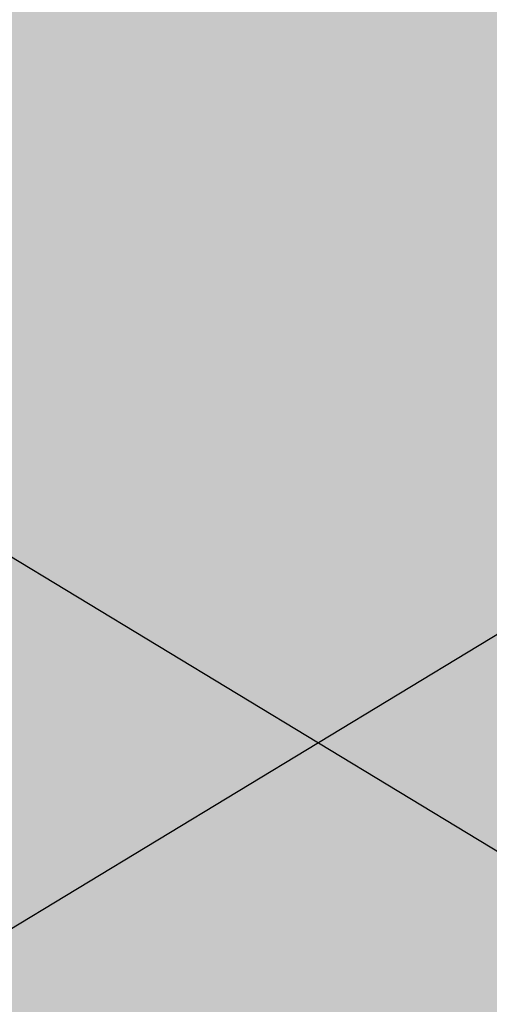
# Model space of a CAD drawing. Units: millimetres. Extents: x -22994 to 29398, y -19990 to 20176.
# Tile 59 of 135: x 215.97 to 223.11, y 79.59 to 94.56. Entities that reach past the tile are written whole.
import ezdxf
from ezdxf import colors
from ezdxf.entities.mleader import LeaderData, LeaderLine
from ezdxf.math import Vec2, Vec3

# ---------------------------------------------------------------- set-up
doc = ezdxf.new("R2010")
doc.units = ezdxf.units.MM
doc.header["$MEASUREMENT"] = 0
for name, color, linetype, lineweight in [('M-ANNO-TEXT', 7, 'Continuous', 25), ('M-DIMS', 2, 'Continuous', 18), ('M-EQPM', 7, 'Continuous', 25), ('M-EQPM-PATT', 7, 'Continuous', 18)]:
    doc.layers.add(name, color=color, linetype=linetype, lineweight=lineweight)
doc.styles.get("Standard").update_dxf_attribs({"font": 'arial.ttf'})
doc.dimstyles.get("Standard").update_dxf_attribs({"dimtxt": 0.18, "dimasz": 10000, "dimexe": 0.18, "dimexo": 0.0625, "dimgap": 0.09, "dimtad": 0, "dimtih": 1, "dimtoh": 1, "dimdec": 0, "dimzin": 0, "dimdsep": 46, "dimtxsty": 'Standard', "dimcen": 0.09, "dimadec": 0, "dimazin": 0, "dimtfac": 1, "dimtdec": 0, "dimtofl": 0, "dimtmove": 0, "dimatfit": 3, "dimfxl": 1, "dimtolj": 1, "dimtzin": 0, "dimlwd": 30, "dimarcsym": 0})

# ---------------------------------------------------------------- blocks, each defined once
blk = doc.blocks.new('*D2')
at = {"layer": 'Defpoints', "color": 0, "transparency": 16777216}
for p in [(6.677, 10.271), (290.852, 10.271), (290.852, -5.079)]:
    blk.add_point(p, dxfattribs=at)
at = {"layer": 'M-DIMS', "color": 0, "lineweight": -2, "transparency": 16777216}
for p, q in [((6.677, 10.209), (6.677, -5.259)), ((290.852, 10.209), (290.852, -5.259))]:
    blk.add_line(p, q, dxfattribs=at)
at = {"layer": 'M-DIMS', "color": 0, "lineweight": 30, "transparency": 16777216}
for p, q in [((-9993.323, -5.079), (-19993.323, -5.079)), ((10290.852, -5.079), (20290.852, -5.079))]:
    blk.add_line(p, q, dxfattribs=at)
at = {"layer": 'M-DIMS', "color": 0, "transparency": 16777216}
for points in [[(-9993.323, 1661.588), (-9993.323, -1671.745), (6.677, -5.079)], [(10290.852, 1661.588), (10290.852, -1671.745), (290.852, -5.079)]]:
    blk.add_solid(points, dxfattribs=at)
at = {"layer": 'M-DIMS', "color": 0, "transparency": 16777216, "insert": (148.765, -5.079), "char_height": 0.18, "attachment_point": 5}
blk.add_mtext('\\A1;284.2', dxfattribs=at)
blk = doc.blocks.new('*D3')
at = {"layer": 'Defpoints', "color": 0, "transparency": 16777216}
for p in [(110.265, 204.165), (110.265, 176.366), (95.833, 127.967)]:
    blk.add_point(p, dxfattribs=at)
at = {"layer": 'M-DIMS', "color": 0, "lineweight": -2, "transparency": 16777216}
for p, q in [((95.833, 128.03), (95.833, 204.345)), ((110.265, 176.429), (110.265, 204.345))]:
    blk.add_line(p, q, dxfattribs=at)
at = {"layer": 'M-DIMS', "color": 0, "lineweight": 30, "transparency": 16777216}
for p, q in [((-9904.167, 204.165), (-19904.167, 204.165)), ((10110.265, 204.165), (20110.265, 204.165))]:
    blk.add_line(p, q, dxfattribs=at)
at = {"layer": 'M-DIMS', "color": 0, "transparency": 16777216}
for points in [[(-9904.167, 1870.832), (-9904.167, -1462.501), (95.833, 204.165)], [(10110.265, 1870.832), (10110.265, -1462.501), (110.265, 204.165)]]:
    blk.add_solid(points, dxfattribs=at)
at = {"layer": 'M-DIMS', "color": 0, "transparency": 16777216, "insert": (103.049, 204.165), "char_height": 0.18, "attachment_point": 5}
blk.add_mtext('\\A1;14.432', dxfattribs=at)
blk = doc.blocks.new('*D4')
at = {"layer": 'Defpoints', "color": 0, "transparency": 16777216}
for p in [(116.265, 204.165), (110.265, 176.366), (116.265, 176.366)]:
    blk.add_point(p, dxfattribs=at)
at = {"layer": 'M-DIMS', "color": 0, "lineweight": -2, "transparency": 16777216}
for p, q in [((110.265, 176.429), (110.265, 204.345)), ((116.265, 176.429), (116.265, 204.345))]:
    blk.add_line(p, q, dxfattribs=at)
at = {"layer": 'M-DIMS', "color": 0, "lineweight": 30, "transparency": 16777216}
for p, q in [((-9889.735, 204.165), (-19889.735, 204.165)), ((10116.265, 204.165), (20116.265, 204.165))]:
    blk.add_line(p, q, dxfattribs=at)
at = {"layer": 'M-DIMS', "color": 0, "transparency": 16777216}
for points in [[(-9889.735, 1870.832), (-9889.735, -1462.501), (110.265, 204.165)], [(10116.265, 1870.832), (10116.265, -1462.501), (116.265, 204.165)]]:
    blk.add_solid(points, dxfattribs=at)
at = {"layer": 'M-DIMS', "color": 0, "transparency": 16777216, "insert": (113.265, 204.165), "char_height": 0.18, "attachment_point": 5}
blk.add_mtext('\\A1;6', dxfattribs=at)
blk = doc.blocks.new('*D5')
at = {"layer": 'Defpoints', "color": 0, "transparency": 16777216}
for p in [(181.265, 204.165), (116.265, 176.366), (181.265, 176.366)]:
    blk.add_point(p, dxfattribs=at)
at = {"layer": 'M-DIMS', "color": 0, "lineweight": -2, "transparency": 16777216}
for p, q in [((116.265, 176.429), (116.265, 204.345)), ((181.265, 176.429), (181.265, 204.345))]:
    blk.add_line(p, q, dxfattribs=at)
at = {"layer": 'M-DIMS', "color": 0, "lineweight": 30, "transparency": 16777216}
for p, q in [((-9883.735, 204.165), (-19883.735, 204.165)), ((10181.265, 204.165), (20181.265, 204.165))]:
    blk.add_line(p, q, dxfattribs=at)
at = {"layer": 'M-DIMS', "color": 0, "transparency": 16777216}
for points in [[(-9883.735, 1870.832), (-9883.735, -1462.501), (116.265, 204.165)], [(10181.265, 1870.832), (10181.265, -1462.501), (181.265, 204.165)]]:
    blk.add_solid(points, dxfattribs=at)
at = {"layer": 'M-DIMS', "color": 0, "transparency": 16777216, "insert": (148.765, 204.165), "char_height": 0.18, "attachment_point": 5}
blk.add_mtext('\\A1;65', dxfattribs=at)
blk = doc.blocks.new('*D6')
at = {"layer": 'Defpoints', "color": 0, "transparency": 16777216}
for p in [(187.265, 204.165), (181.265, 176.366), (187.265, 176.366)]:
    blk.add_point(p, dxfattribs=at)
at = {"layer": 'M-DIMS', "color": 0, "lineweight": -2, "transparency": 16777216}
for p, q in [((181.265, 176.429), (181.265, 204.345)), ((187.265, 176.429), (187.265, 204.345))]:
    blk.add_line(p, q, dxfattribs=at)
at = {"layer": 'M-DIMS', "color": 0, "lineweight": 30, "transparency": 16777216}
for p, q in [((-9818.735, 204.165), (-19818.735, 204.165)), ((10187.265, 204.165), (20187.265, 204.165))]:
    blk.add_line(p, q, dxfattribs=at)
at = {"layer": 'M-DIMS', "color": 0, "transparency": 16777216}
for points in [[(-9818.735, 1870.832), (-9818.735, -1462.501), (181.265, 204.165)], [(10187.265, 1870.832), (10187.265, -1462.501), (187.265, 204.165)]]:
    blk.add_solid(points, dxfattribs=at)
at = {"layer": 'M-DIMS', "color": 0, "transparency": 16777216, "insert": (184.265, 204.165), "char_height": 0.18, "attachment_point": 5}
blk.add_mtext('\\A1;6', dxfattribs=at)
blk = doc.blocks.new('*D7')
at = {"layer": 'Defpoints', "color": 0, "transparency": 16777216}
for p in [(201.697, 204.165), (187.265, 176.366), (201.697, 127.967)]:
    blk.add_point(p, dxfattribs=at)
at = {"layer": 'M-DIMS', "color": 0, "lineweight": -2, "transparency": 16777216}
for p, q in [((187.265, 176.429), (187.265, 204.345)), ((201.697, 128.03), (201.697, 204.345))]:
    blk.add_line(p, q, dxfattribs=at)
at = {"layer": 'M-DIMS', "color": 0, "lineweight": 30, "transparency": 16777216}
for p, q in [((-9812.735, 204.165), (-19812.735, 204.165)), ((10201.697, 204.165), (20201.697, 204.165))]:
    blk.add_line(p, q, dxfattribs=at)
at = {"layer": 'M-DIMS', "color": 0, "transparency": 16777216}
for points in [[(-9812.735, 1870.832), (-9812.735, -1462.501), (187.265, 204.165)], [(10201.697, 1870.832), (10201.697, -1462.501), (201.697, 204.165)]]:
    blk.add_solid(points, dxfattribs=at)
at = {"layer": 'M-DIMS', "color": 0, "transparency": 16777216, "insert": (194.481, 204.165), "char_height": 0.18, "attachment_point": 5}
blk.add_mtext('\\A1;14.432', dxfattribs=at)
blk = doc.blocks.new('*D8')
at = {"layer": 'Defpoints', "color": 0, "transparency": 16777216}
for p in [(227.648, 204.165), (227.648, 146.73), (201.697, 127.967)]:
    blk.add_point(p, dxfattribs=at)
at = {"layer": 'M-DIMS', "color": 0, "lineweight": -2, "transparency": 16777216}
for p, q in [((201.697, 128.03), (201.697, 204.345)), ((227.648, 146.792), (227.648, 204.345))]:
    blk.add_line(p, q, dxfattribs=at)
at = {"layer": 'M-DIMS', "color": 0, "lineweight": 30, "transparency": 16777216}
for p, q in [((-9798.303, 204.165), (-19798.303, 204.165)), ((10227.648, 204.165), (20227.648, 204.165))]:
    blk.add_line(p, q, dxfattribs=at)
at = {"layer": 'M-DIMS', "color": 0, "transparency": 16777216}
for points in [[(-9798.303, 1870.832), (-9798.303, -1462.501), (201.697, 204.165)], [(10227.648, 1870.832), (10227.648, -1462.501), (227.648, 204.165)]]:
    blk.add_solid(points, dxfattribs=at)
at = {"layer": 'M-DIMS', "color": 0, "transparency": 16777216, "insert": (214.673, 204.165), "char_height": 0.18, "attachment_point": 5}
blk.add_mtext('\\A1;25.95', dxfattribs=at)
blk = doc.blocks.new('*D9')
at = {"layer": 'Defpoints', "color": 0, "transparency": 16777216}
for p in [(187.265, 176.366), (306.202, 176.366), (290.852, 10.271)]:
    blk.add_point(p, dxfattribs=at)
at = {"layer": 'M-DIMS', "color": 0, "lineweight": 30, "transparency": 16777216}
for p, q in [((306.202, 10176.366), (306.202, 20176.366)), ((306.202, -9989.729), (306.202, -19989.729))]:
    blk.add_line(p, q, dxfattribs=at)
at = {"layer": 'M-DIMS', "color": 0, "lineweight": -2, "transparency": 16777216}
for p, q in [((187.327, 176.366), (306.382, 176.366)), ((290.915, 10.271), (306.382, 10.271))]:
    blk.add_line(p, q, dxfattribs=at)
at = {"layer": 'M-DIMS', "color": 0, "transparency": 16777216}
for points in [[(-1360.465, 10176.366), (1972.869, 10176.366), (306.202, 176.366)], [(-1360.465, -9989.729), (1972.869, -9989.729), (306.202, 10.271)]]:
    blk.add_solid(points, dxfattribs=at)
at = {"layer": 'M-DIMS', "color": 0, "transparency": 16777216, "insert": (306.202, 93.319), "char_height": 0.18, "attachment_point": 5}
blk.add_mtext('\\A1;166.1', dxfattribs=at)
blk = doc.blocks.new('*D10')
at = {"layer": 'Defpoints', "color": 0, "transparency": 16777216}
for p in [(125.65, 136.071), (133.346, 136.071), (133.346, -5.079)]:
    blk.add_point(p, dxfattribs=at)
at = {"layer": 'M-DIMS', "color": 0, "lineweight": -2, "transparency": 16777216}
for p, q in [((125.65, 136.009), (125.65, -5.259)), ((133.346, 136.009), (133.346, -5.259))]:
    blk.add_line(p, q, dxfattribs=at)
at = {"layer": 'M-DIMS', "color": 0, "lineweight": 30, "transparency": 16777216}
for p, q in [((-9874.35, -5.079), (-19874.35, -5.079)), ((10133.346, -5.079), (20133.346, -5.079))]:
    blk.add_line(p, q, dxfattribs=at)
at = {"layer": 'M-DIMS', "color": 0, "transparency": 16777216}
for points in [[(-9874.35, 1661.588), (-9874.35, -1671.745), (125.65, -5.079)], [(10133.346, 1661.588), (10133.346, -1671.745), (133.346, -5.079)]]:
    blk.add_solid(points, dxfattribs=at)
at = {"layer": 'M-DIMS', "color": 0, "transparency": 16777216, "insert": (129.498, -5.079), "char_height": 0.18, "attachment_point": 5}
blk.add_mtext('\\A1;7.696', dxfattribs=at)
blk = doc.blocks.new('*D11')
at = {"layer": 'Defpoints', "color": 0, "transparency": 16777216}
for p in [(133.346, 136.071), (135.65, 136.071), (135.65, -5.079)]:
    blk.add_point(p, dxfattribs=at)
at = {"layer": 'M-DIMS', "color": 0, "lineweight": -2, "transparency": 16777216}
for p, q in [((133.346, 136.009), (133.346, -5.259)), ((135.65, 136.009), (135.65, -5.259))]:
    blk.add_line(p, q, dxfattribs=at)
at = {"layer": 'M-DIMS', "color": 0, "lineweight": 30, "transparency": 16777216}
for p, q in [((-9866.654, -5.079), (-19866.654, -5.079)), ((10135.65, -5.079), (20135.65, -5.079))]:
    blk.add_line(p, q, dxfattribs=at)
at = {"layer": 'M-DIMS', "color": 0, "transparency": 16777216}
for points in [[(-9866.654, 1661.588), (-9866.654, -1671.745), (133.346, -5.079)], [(10135.65, 1661.588), (10135.65, -1671.745), (135.65, -5.079)]]:
    blk.add_solid(points, dxfattribs=at)
at = {"layer": 'M-DIMS', "color": 0, "transparency": 16777216, "insert": (134.498, -5.079), "char_height": 0.18, "attachment_point": 5}
blk.add_mtext('\\A1;2.304', dxfattribs=at)
blk = doc.blocks.new('*D12')
at = {"layer": 'Defpoints', "color": 0, "transparency": 16777216}
for p in [(135.65, 136.071), (145.65, 136.071), (145.65, -5.079)]:
    blk.add_point(p, dxfattribs=at)
at = {"layer": 'M-DIMS', "color": 0, "lineweight": -2, "transparency": 16777216}
for p, q in [((135.65, 136.009), (135.65, -5.259)), ((145.65, 136.009), (145.65, -5.259))]:
    blk.add_line(p, q, dxfattribs=at)
at = {"layer": 'M-DIMS', "color": 0, "lineweight": 30, "transparency": 16777216}
for p, q in [((-9864.35, -5.079), (-19864.35, -5.079)), ((10145.65, -5.079), (20145.65, -5.079))]:
    blk.add_line(p, q, dxfattribs=at)
at = {"layer": 'M-DIMS', "color": 0, "transparency": 16777216}
for points in [[(-9864.35, 1661.588), (-9864.35, -1671.745), (135.65, -5.079)], [(10145.65, 1661.588), (10145.65, -1671.745), (145.65, -5.079)]]:
    blk.add_solid(points, dxfattribs=at)
at = {"layer": 'M-DIMS', "color": 0, "transparency": 16777216, "insert": (140.65, -5.079), "char_height": 0.18, "attachment_point": 5}
blk.add_mtext('\\A1;10', dxfattribs=at)
blk = doc.blocks.new('*D13')
at = {"layer": 'Defpoints', "color": 0, "transparency": 16777216}
for p in [(145.65, 136.071), (155.65, 136.071), (155.65, -5.079)]:
    blk.add_point(p, dxfattribs=at)
at = {"layer": 'M-DIMS', "color": 0, "lineweight": -2, "transparency": 16777216}
for p, q in [((145.65, 136.009), (145.65, -5.259)), ((155.65, 136.009), (155.65, -5.259))]:
    blk.add_line(p, q, dxfattribs=at)
at = {"layer": 'M-DIMS', "color": 0, "lineweight": 30, "transparency": 16777216}
for p, q in [((-9854.35, -5.079), (-19854.35, -5.079)), ((10155.65, -5.079), (20155.65, -5.079))]:
    blk.add_line(p, q, dxfattribs=at)
at = {"layer": 'M-DIMS', "color": 0, "transparency": 16777216}
for points in [[(-9854.35, 1661.588), (-9854.35, -1671.745), (145.65, -5.079)], [(10155.65, 1661.588), (10155.65, -1671.745), (155.65, -5.079)]]:
    blk.add_solid(points, dxfattribs=at)
at = {"layer": 'M-DIMS', "color": 0, "transparency": 16777216, "insert": (150.65, -5.079), "char_height": 0.18, "attachment_point": 5}
blk.add_mtext('\\A1;10', dxfattribs=at)
blk = doc.blocks.new('*D14')
at = {"layer": 'Defpoints', "color": 0, "transparency": 16777216}
for p in [(155.65, 136.071), (165.65, 136.071), (165.65, -5.079)]:
    blk.add_point(p, dxfattribs=at)
at = {"layer": 'M-DIMS', "color": 0, "lineweight": -2, "transparency": 16777216}
for p, q in [((155.65, 136.009), (155.65, -5.259)), ((165.65, 136.009), (165.65, -5.259))]:
    blk.add_line(p, q, dxfattribs=at)
at = {"layer": 'M-DIMS', "color": 0, "lineweight": 30, "transparency": 16777216}
for p, q in [((-9844.35, -5.079), (-19844.35, -5.079)), ((10165.65, -5.079), (20165.65, -5.079))]:
    blk.add_line(p, q, dxfattribs=at)
at = {"layer": 'M-DIMS', "color": 0, "transparency": 16777216}
for points in [[(-9844.35, 1661.588), (-9844.35, -1671.745), (155.65, -5.079)], [(10165.65, 1661.588), (10165.65, -1671.745), (165.65, -5.079)]]:
    blk.add_solid(points, dxfattribs=at)
at = {"layer": 'M-DIMS', "color": 0, "transparency": 16777216, "insert": (160.65, -5.079), "char_height": 0.18, "attachment_point": 5}
blk.add_mtext('\\A1;10', dxfattribs=at)
blk = doc.blocks.new('*D15')
at = {"layer": 'Defpoints', "color": 0, "transparency": 16777216}
for p in [(173.346, 154.788), (173.346, 136.071), (306.202, 136.071)]:
    blk.add_point(p, dxfattribs=at)
at = {"layer": 'M-DIMS', "color": 0, "lineweight": 30, "transparency": 16777216}
for p, q in [((306.202, 10154.788), (306.202, 20154.788)), ((306.202, -9863.929), (306.202, -19863.929))]:
    blk.add_line(p, q, dxfattribs=at)
at = {"layer": 'M-DIMS', "color": 0, "lineweight": -2, "transparency": 16777216}
for p, q in [((173.408, 154.788), (306.382, 154.788)), ((173.408, 136.071), (306.382, 136.071))]:
    blk.add_line(p, q, dxfattribs=at)
at = {"layer": 'M-DIMS', "color": 0, "transparency": 16777216}
for points in [[(-1360.465, 10154.788), (1972.869, 10154.788), (306.202, 154.788)], [(-1360.465, -9863.929), (1972.869, -9863.929), (306.202, 136.071)]]:
    blk.add_solid(points, dxfattribs=at)
at = {"layer": 'M-DIMS', "color": 0, "transparency": 16777216, "insert": (306.202, 145.43), "char_height": 0.18, "attachment_point": 5}
blk.add_mtext('\\A1;18.717', dxfattribs=at)
blk = doc.blocks.new('*D16')
at = {"layer": 'Defpoints', "color": 0, "transparency": 16777216}
for p in [(120.17, 204.165), (110.466, 48.035), (120.17, 48.035)]:
    blk.add_point(p, dxfattribs=at)
at = {"layer": 'M-DIMS', "color": 0, "lineweight": -2, "transparency": 16777216}
for p, q in [((110.466, 48.097), (110.466, 204.345)), ((120.17, 48.097), (120.17, 204.345))]:
    blk.add_line(p, q, dxfattribs=at)
at = {"layer": 'M-DIMS', "color": 0, "lineweight": 30, "transparency": 16777216}
for p, q in [((-9889.534, 204.165), (-19889.534, 204.165)), ((10120.17, 204.165), (20120.17, 204.165))]:
    blk.add_line(p, q, dxfattribs=at)
at = {"layer": 'M-DIMS', "color": 0, "transparency": 16777216}
for points in [[(-9889.534, 1870.832), (-9889.534, -1462.501), (110.466, 204.165)], [(10120.17, 1870.832), (10120.17, -1462.501), (120.17, 204.165)]]:
    blk.add_solid(points, dxfattribs=at)
at = {"layer": 'M-DIMS', "color": 0, "transparency": 16777216, "insert": (115.318, 204.165), "char_height": 0.18, "attachment_point": 5}
blk.add_mtext('\\A1;9.704', dxfattribs=at)
blk = doc.blocks.new('*D17')
at = {"layer": 'Defpoints', "color": 0, "transparency": 16777216}
for p in [(126.17, 204.165), (120.17, 48.035), (126.17, 48.035)]:
    blk.add_point(p, dxfattribs=at)
at = {"layer": 'M-DIMS', "color": 0, "lineweight": -2, "transparency": 16777216}
for p, q in [((120.17, 48.097), (120.17, 204.345)), ((126.17, 48.097), (126.17, 204.345))]:
    blk.add_line(p, q, dxfattribs=at)
at = {"layer": 'M-DIMS', "color": 0, "lineweight": 30, "transparency": 16777216}
for p, q in [((-9879.83, 204.165), (-19879.83, 204.165)), ((10126.17, 204.165), (20126.17, 204.165))]:
    blk.add_line(p, q, dxfattribs=at)
at = {"layer": 'M-DIMS', "color": 0, "transparency": 16777216}
for points in [[(-9879.83, 1870.832), (-9879.83, -1462.501), (120.17, 204.165)], [(10126.17, 1870.832), (10126.17, -1462.501), (126.17, 204.165)]]:
    blk.add_solid(points, dxfattribs=at)
at = {"layer": 'M-DIMS', "color": 0, "transparency": 16777216, "insert": (123.17, 204.165), "char_height": 0.18, "attachment_point": 5}
blk.add_mtext('\\A1;6', dxfattribs=at)
blk = doc.blocks.new('*D18')
at = {"layer": 'Defpoints', "color": 0, "transparency": 16777216}
for p in [(132.17, 204.165), (126.17, 48.035), (132.17, 48.035)]:
    blk.add_point(p, dxfattribs=at)
at = {"layer": 'M-DIMS', "color": 0, "lineweight": -2, "transparency": 16777216}
for p, q in [((126.17, 48.097), (126.17, 204.345)), ((132.17, 48.097), (132.17, 204.345))]:
    blk.add_line(p, q, dxfattribs=at)
at = {"layer": 'M-DIMS', "color": 0, "lineweight": 30, "transparency": 16777216}
for p, q in [((-9873.83, 204.165), (-19873.83, 204.165)), ((10132.17, 204.165), (20132.17, 204.165))]:
    blk.add_line(p, q, dxfattribs=at)
at = {"layer": 'M-DIMS', "color": 0, "transparency": 16777216}
for points in [[(-9873.83, 1870.832), (-9873.83, -1462.501), (126.17, 204.165)], [(10132.17, 1870.832), (10132.17, -1462.501), (132.17, 204.165)]]:
    blk.add_solid(points, dxfattribs=at)
at = {"layer": 'M-DIMS', "color": 0, "transparency": 16777216, "insert": (129.17, 204.165), "char_height": 0.18, "attachment_point": 5}
blk.add_mtext('\\A1;6', dxfattribs=at)
blk = doc.blocks.new('*D19')
at = {"layer": 'Defpoints', "color": 0, "transparency": 16777216}
for p in [(138.17, 204.165), (132.17, 48.035), (138.17, 48.035)]:
    blk.add_point(p, dxfattribs=at)
at = {"layer": 'M-DIMS', "color": 0, "lineweight": -2, "transparency": 16777216}
for p, q in [((132.17, 48.097), (132.17, 204.345)), ((138.17, 48.097), (138.17, 204.345))]:
    blk.add_line(p, q, dxfattribs=at)
at = {"layer": 'M-DIMS', "color": 0, "lineweight": 30, "transparency": 16777216}
for p, q in [((-9867.83, 204.165), (-19867.83, 204.165)), ((10138.17, 204.165), (20138.17, 204.165))]:
    blk.add_line(p, q, dxfattribs=at)
at = {"layer": 'M-DIMS', "color": 0, "transparency": 16777216}
for points in [[(-9867.83, 1870.832), (-9867.83, -1462.501), (132.17, 204.165)], [(10138.17, 1870.832), (10138.17, -1462.501), (138.17, 204.165)]]:
    blk.add_solid(points, dxfattribs=at)
at = {"layer": 'M-DIMS', "color": 0, "transparency": 16777216, "insert": (135.17, 204.165), "char_height": 0.18, "attachment_point": 5}
blk.add_mtext('\\A1;6', dxfattribs=at)
blk = doc.blocks.new('*D20')
at = {"layer": 'Defpoints', "color": 0, "transparency": 16777216}
for p in [(144.17, 204.165), (138.17, 48.035), (144.17, 48.035)]:
    blk.add_point(p, dxfattribs=at)
at = {"layer": 'M-DIMS', "color": 0, "lineweight": -2, "transparency": 16777216}
for p, q in [((138.17, 48.097), (138.17, 204.345)), ((144.17, 48.097), (144.17, 204.345))]:
    blk.add_line(p, q, dxfattribs=at)
at = {"layer": 'M-DIMS', "color": 0, "lineweight": 30, "transparency": 16777216}
for p, q in [((-9861.83, 204.165), (-19861.83, 204.165)), ((10144.17, 204.165), (20144.17, 204.165))]:
    blk.add_line(p, q, dxfattribs=at)
at = {"layer": 'M-DIMS', "color": 0, "transparency": 16777216}
for points in [[(-9861.83, 1870.832), (-9861.83, -1462.501), (138.17, 204.165)], [(10144.17, 1870.832), (10144.17, -1462.501), (144.17, 204.165)]]:
    blk.add_solid(points, dxfattribs=at)
at = {"layer": 'M-DIMS', "color": 0, "transparency": 16777216, "insert": (141.17, 204.165), "char_height": 0.18, "attachment_point": 5}
blk.add_mtext('\\A1;6', dxfattribs=at)
blk = doc.blocks.new('*D21')
at = {"layer": 'Defpoints', "color": 0, "transparency": 16777216}
for p in [(149.116, 204.165), (144.17, 48.035), (149.116, 48.035)]:
    blk.add_point(p, dxfattribs=at)
at = {"layer": 'M-DIMS', "color": 0, "lineweight": -2, "transparency": 16777216}
for p, q in [((144.17, 48.097), (144.17, 204.345)), ((149.116, 48.097), (149.116, 204.345))]:
    blk.add_line(p, q, dxfattribs=at)
at = {"layer": 'M-DIMS', "color": 0, "lineweight": 30, "transparency": 16777216}
for p, q in [((-9855.83, 204.165), (-19855.83, 204.165)), ((10149.116, 204.165), (20149.116, 204.165))]:
    blk.add_line(p, q, dxfattribs=at)
at = {"layer": 'M-DIMS', "color": 0, "transparency": 16777216}
for points in [[(-9855.83, 1870.832), (-9855.83, -1462.501), (144.17, 204.165)], [(10149.116, 1870.832), (10149.116, -1462.501), (149.116, 204.165)]]:
    blk.add_solid(points, dxfattribs=at)
at = {"layer": 'M-DIMS', "color": 0, "transparency": 16777216, "insert": (146.643, 204.165), "char_height": 0.18, "attachment_point": 5}
blk.add_mtext('\\A1;4.945', dxfattribs=at)
blk = doc.blocks.new('*D22')
at = {"layer": 'Defpoints', "color": 0, "transparency": 16777216}
for p in [(149.116, 30.99), (155.116, 30.99), (155.116, -5.079)]:
    blk.add_point(p, dxfattribs=at)
at = {"layer": 'M-DIMS', "color": 0, "lineweight": -2, "transparency": 16777216}
for p, q in [((149.116, 30.927), (149.116, -5.259)), ((155.116, 30.927), (155.116, -5.259))]:
    blk.add_line(p, q, dxfattribs=at)
at = {"layer": 'M-DIMS', "color": 0, "lineweight": 30, "transparency": 16777216}
for p, q in [((-9850.884, -5.079), (-19850.884, -5.079)), ((10155.116, -5.079), (20155.116, -5.079))]:
    blk.add_line(p, q, dxfattribs=at)
at = {"layer": 'M-DIMS', "color": 0, "transparency": 16777216}
for points in [[(-9850.884, 1661.588), (-9850.884, -1671.745), (149.116, -5.079)], [(10155.116, 1661.588), (10155.116, -1671.745), (155.116, -5.079)]]:
    blk.add_solid(points, dxfattribs=at)
at = {"layer": 'M-DIMS', "color": 0, "transparency": 16777216, "insert": (152.116, -5.079), "char_height": 0.18, "attachment_point": 5}
blk.add_mtext('\\A1;6', dxfattribs=at)
blk = doc.blocks.new('*D23')
at = {"layer": 'Defpoints', "color": 0, "transparency": 16777216}
for p in [(155.116, 30.99), (161.116, 30.99), (161.116, -5.079)]:
    blk.add_point(p, dxfattribs=at)
at = {"layer": 'M-DIMS', "color": 0, "lineweight": -2, "transparency": 16777216}
for p, q in [((155.116, 30.927), (155.116, -5.259)), ((161.116, 30.927), (161.116, -5.259))]:
    blk.add_line(p, q, dxfattribs=at)
at = {"layer": 'M-DIMS', "color": 0, "lineweight": 30, "transparency": 16777216}
for p, q in [((-9844.884, -5.079), (-19844.884, -5.079)), ((10161.116, -5.079), (20161.116, -5.079))]:
    blk.add_line(p, q, dxfattribs=at)
at = {"layer": 'M-DIMS', "color": 0, "transparency": 16777216}
for points in [[(-9844.884, 1661.588), (-9844.884, -1671.745), (155.116, -5.079)], [(10161.116, 1661.588), (10161.116, -1671.745), (161.116, -5.079)]]:
    blk.add_solid(points, dxfattribs=at)
at = {"layer": 'M-DIMS', "color": 0, "transparency": 16777216, "insert": (158.116, -5.079), "char_height": 0.18, "attachment_point": 5}
blk.add_mtext('\\A1;6', dxfattribs=at)
blk = doc.blocks.new('*D24')
at = {"layer": 'Defpoints', "color": 0, "transparency": 16777216}
for p in [(161.116, 30.99), (166.439, 30.99), (166.439, -5.079)]:
    blk.add_point(p, dxfattribs=at)
at = {"layer": 'M-DIMS', "color": 0, "lineweight": -2, "transparency": 16777216}
for p, q in [((161.116, 30.927), (161.116, -5.259)), ((166.439, 30.927), (166.439, -5.259))]:
    blk.add_line(p, q, dxfattribs=at)
at = {"layer": 'M-DIMS', "color": 0, "lineweight": 30, "transparency": 16777216}
for p, q in [((-9838.884, -5.079), (-19838.884, -5.079)), ((10166.439, -5.079), (20166.439, -5.079))]:
    blk.add_line(p, q, dxfattribs=at)
at = {"layer": 'M-DIMS', "color": 0, "transparency": 16777216}
for points in [[(-9838.884, 1661.588), (-9838.884, -1671.745), (161.116, -5.079)], [(10166.439, 1661.588), (10166.439, -1671.745), (166.439, -5.079)]]:
    blk.add_solid(points, dxfattribs=at)
at = {"layer": 'M-DIMS', "color": 0, "transparency": 16777216, "insert": (163.777, -5.079), "char_height": 0.18, "attachment_point": 5}
blk.add_mtext('\\A1;5.323', dxfattribs=at)
blk = doc.blocks.new('*D25')
at = {"layer": 'Defpoints', "color": 0, "transparency": 16777216}
for p in [(166.439, 30.99), (172.439, 30.99), (172.439, -5.079)]:
    blk.add_point(p, dxfattribs=at)
at = {"layer": 'M-DIMS', "color": 0, "lineweight": -2, "transparency": 16777216}
for p, q in [((166.439, 30.927), (166.439, -5.259)), ((172.439, 30.927), (172.439, -5.259))]:
    blk.add_line(p, q, dxfattribs=at)
at = {"layer": 'M-DIMS', "color": 0, "lineweight": 30, "transparency": 16777216}
for p, q in [((-9833.561, -5.079), (-19833.561, -5.079)), ((10172.439, -5.079), (20172.439, -5.079))]:
    blk.add_line(p, q, dxfattribs=at)
at = {"layer": 'M-DIMS', "color": 0, "transparency": 16777216}
for points in [[(-9833.561, 1661.588), (-9833.561, -1671.745), (166.439, -5.079)], [(10172.439, 1661.588), (10172.439, -1671.745), (172.439, -5.079)]]:
    blk.add_solid(points, dxfattribs=at)
at = {"layer": 'M-DIMS', "color": 0, "transparency": 16777216, "insert": (169.439, -5.079), "char_height": 0.18, "attachment_point": 5}
blk.add_mtext('\\A1;6', dxfattribs=at)
blk = doc.blocks.new('*D26')
at = {"layer": 'Defpoints', "color": 0, "transparency": 16777216}
for p in [(172.439, 30.99), (178.439, 30.99), (178.439, -5.079)]:
    blk.add_point(p, dxfattribs=at)
at = {"layer": 'M-DIMS', "color": 0, "lineweight": -2, "transparency": 16777216}
for p, q in [((172.439, 30.927), (172.439, -5.259)), ((178.439, 30.927), (178.439, -5.259))]:
    blk.add_line(p, q, dxfattribs=at)
at = {"layer": 'M-DIMS', "color": 0, "lineweight": 30, "transparency": 16777216}
for p, q in [((-9827.561, -5.079), (-19827.561, -5.079)), ((10178.439, -5.079), (20178.439, -5.079))]:
    blk.add_line(p, q, dxfattribs=at)
at = {"layer": 'M-DIMS', "color": 0, "transparency": 16777216}
for points in [[(-9827.561, 1661.588), (-9827.561, -1671.745), (172.439, -5.079)], [(10178.439, 1661.588), (10178.439, -1671.745), (178.439, -5.079)]]:
    blk.add_solid(points, dxfattribs=at)
at = {"layer": 'M-DIMS', "color": 0, "transparency": 16777216, "insert": (175.439, -5.079), "char_height": 0.18, "attachment_point": 5}
blk.add_mtext('\\A1;6', dxfattribs=at)
blk = doc.blocks.new('*D27')
at = {"layer": 'Defpoints', "color": 0, "transparency": 16777216}
for p in [(178.439, 30.99), (188.117, 30.99), (188.117, -5.079)]:
    blk.add_point(p, dxfattribs=at)
at = {"layer": 'M-DIMS', "color": 0, "lineweight": -2, "transparency": 16777216}
for p, q in [((178.439, 30.927), (178.439, -5.259)), ((188.117, 30.927), (188.117, -5.259))]:
    blk.add_line(p, q, dxfattribs=at)
at = {"layer": 'M-DIMS', "color": 0, "lineweight": 30, "transparency": 16777216}
for p, q in [((-9821.561, -5.079), (-19821.561, -5.079)), ((10188.117, -5.079), (20188.117, -5.079))]:
    blk.add_line(p, q, dxfattribs=at)
at = {"layer": 'M-DIMS', "color": 0, "transparency": 16777216}
for points in [[(-9821.561, 1661.588), (-9821.561, -1671.745), (178.439, -5.079)], [(10188.117, 1661.588), (10188.117, -1671.745), (188.117, -5.079)]]:
    blk.add_solid(points, dxfattribs=at)
at = {"layer": 'M-DIMS', "color": 0, "transparency": 16777216, "insert": (183.278, -5.079), "char_height": 0.18, "attachment_point": 5}
blk.add_mtext('\\A1;9.679', dxfattribs=at)
blk = doc.blocks.new('*D28')
at = {"layer": 'Defpoints', "color": 0, "transparency": 16777216}
for p in [(188.117, 48.035), (306.202, 48.035), (188.117, 30.99)]:
    blk.add_point(p, dxfattribs=at)
at = {"layer": 'M-DIMS', "color": 0, "lineweight": 30, "transparency": 16777216}
for p, q in [((306.202, 10048.035), (306.202, 20048.035)), ((306.202, -9969.01), (306.202, -19969.01))]:
    blk.add_line(p, q, dxfattribs=at)
at = {"layer": 'M-DIMS', "color": 0, "lineweight": -2, "transparency": 16777216}
for p, q in [((188.18, 48.035), (306.382, 48.035)), ((188.18, 30.99), (306.382, 30.99))]:
    blk.add_line(p, q, dxfattribs=at)
at = {"layer": 'M-DIMS', "color": 0, "transparency": 16777216}
for points in [[(-1360.465, 10048.035), (1972.869, 10048.035), (306.202, 48.035)], [(-1360.465, -9969.01), (1972.869, -9969.01), (306.202, 30.99)]]:
    blk.add_solid(points, dxfattribs=at)
at = {"layer": 'M-DIMS', "color": 0, "transparency": 16777216, "insert": (306.202, 39.512), "char_height": 0.18, "attachment_point": 5}
blk.add_mtext('\\A1;17.045', dxfattribs=at)
blk = doc.blocks.new('*D29')
at = {"layer": 'Defpoints', "color": 0, "transparency": 16777216}
for p in [(36.801, 80.045), (64.03, 80.045)]:
    blk.add_point(p, dxfattribs=at)
at = {"layer": 'M-DIMS', "color": 0, "lineweight": -2, "transparency": 16777216}
for p, q in [((50.415, 79.955), (50.415, 80.135)), ((50.325, 80.045), (50.505, 80.045))]:
    blk.add_line(p, q, dxfattribs=at)
at = {"layer": 'M-DIMS', "color": 0, "lineweight": 30, "transparency": 16777216}
blk.add_line((20064.03, 80.03), (10064.03, 80.038), dxfattribs=at)
at = {"layer": 'M-DIMS', "color": 0, "transparency": 16777216}
blk.add_solid([(10064.031, 1746.704), (10064.028, -1586.629), (64.03, 80.045)], dxfattribs=at)
at = {"layer": 'M-DIMS', "color": 0, "transparency": 16777216, "insert": (20064.521, 80.03), "char_height": 0.18, "attachment_point": 5}
blk.add_mtext('\\A1;∅27.23', dxfattribs=at)
blk = doc.blocks.new('*D30')
at = {"layer": 'Defpoints', "color": 0, "transparency": 16777216}
for p in [(216.315, 146.729), (238.982, 146.73)]:
    blk.add_point(p, dxfattribs=at)
at = {"layer": 'M-DIMS', "color": 0, "lineweight": 30, "transparency": 16777216}
blk.add_line((20238.982, 147.496), (10238.982, 147.113), dxfattribs=at)
at = {"layer": 'M-DIMS', "color": 0, "lineweight": -2, "transparency": 16777216}
for p, q in [((227.558, 146.73), (227.738, 146.73)), ((227.648, 146.64), (227.648, 146.82))]:
    blk.add_line(p, q, dxfattribs=at)
at = {"layer": 'M-DIMS', "color": 0, "transparency": 16777216}
blk.add_solid([(10238.918, 1813.78), (10239.046, -1519.554), (238.982, 146.73)], dxfattribs=at)
at = {"layer": 'M-DIMS', "color": 0, "transparency": 16777216, "insert": (20239.544, 147.496), "char_height": 0.18, "attachment_point": 5}
blk.add_mtext('\\A1;∅22.667', dxfattribs=at)
blk = doc.blocks.new('*D36')
at = {"layer": 'Defpoints', "color": 0, "transparency": 16777216}
for p in [(46.39, 31.303), (46.387, 26.593)]:
    blk.add_point(p, dxfattribs=at)
at = {"layer": 'M-DIMS', "color": 0, "lineweight": 30, "transparency": 16777216}
for p, q in [((57.15, 20031.301), (51.77, 10031.302)), ((10057.15, 20031.301), (57.15, 20031.301))]:
    blk.add_line(p, q, dxfattribs=at)
at = {"layer": 'M-DIMS', "color": 0, "lineweight": -2, "transparency": 16777216}
for p, q in [((46.299, 28.948), (46.479, 28.948)), ((46.389, 28.858), (46.389, 29.038))]:
    blk.add_line(p, q, dxfattribs=at)
at = {"layer": 'M-DIMS', "color": 0, "transparency": 16777216}
blk.add_solid([(-1614.896, 10032.199), (1718.436, 10030.405), (46.39, 31.303)], dxfattribs=at)
at = {"layer": 'M-DIMS', "color": 0, "transparency": 16777216, "insert": (10057.554, 20031.301), "char_height": 0.18, "attachment_point": 5}
blk.add_mtext('\\A1;∅4.71', dxfattribs=at)
blk = doc.blocks.new('*D37')
at = {"layer": 'Defpoints', "color": 0, "transparency": 16777216}
for p in [(54.834, 118.615), (59.494, 118.614)]:
    blk.add_point(p, dxfattribs=at)
at = {"layer": 'M-DIMS', "color": 0, "lineweight": -2, "transparency": 16777216}
for p, q in [((57.074, 118.614), (57.254, 118.614)), ((57.164, 118.524), (57.164, 118.704))]:
    blk.add_line(p, q, dxfattribs=at)
at = {"layer": 'M-DIMS', "color": 0, "lineweight": 30, "transparency": 16777216}
blk.add_line((20059.493, 116.253), (10059.494, 117.434), dxfattribs=at)
at = {"layer": 'M-DIMS', "color": 0, "transparency": 16777216}
blk.add_solid([(10059.69, 1784.1), (10059.297, -1549.233), (59.494, 118.614)], dxfattribs=at)
at = {"layer": 'M-DIMS', "color": 0, "transparency": 16777216, "insert": (20059.985, 116.253), "char_height": 0.18, "attachment_point": 5}
blk.add_mtext('\\A1;∅4.659', dxfattribs=at)

msp = doc.modelspace()

# ---------------------------------------------------------------- hatches: boundary and pattern name
at = {"layer": 'M-EQPM-PATT'}
h = msp.add_hatch(color=256, dxfattribs=at)
h.set_gradient(color1=(205, 32, 39), color2=(205, 32, 39), tint=1)
h.paths.add_polyline_path([(116.2647, 150.3662), (116.2647, 170.3662), (116.2647, 176.3662), (110.2647, 176.3662), (110.2647, 152.0276), (95.8327, 127.967), (95.8327, 16.6063), (201.6967, 16.6063), (201.6967, 127.967), (187.2647, 152.0276), (187.2647, 176.3662), (181.2647, 176.3662), (181.2647, 170.3662), (181.2647, 150.3662), (195.6967, 126.3055), (195.6967, 22.6063), (101.8327, 22.6063), (101.8327, 126.3055)])
h.paths.add_polyline_path([(185.2208, 88.6347), (101.8327, 88.6347), (101.8327, 87.6347), (182.8066, 87.6347), (178.7313, 83.5594), (195.6967, 83.5594), (195.6967, 84.5594), (181.1455, 84.5594)], flags=17)
h.paths.add_polyline_path([(95.8327, 88.6347), (60.9779, 88.6347, -0.0228552), (61.7178, 87.6347), (95.8327, 87.6347)])
h.paths.add_polyline_path([(215.6212, 86.5189), (215.6212, 80.5999), (220.5095, 83.5594)])
h.paths.add_polyline_path([(215.6212, 84.5594), (201.6967, 84.5594), (201.6967, 83.5594), (215.6212, 83.5594)])
h.paths.add_polyline_path([(225.3978, 86.5189), (220.5095, 83.5594), (225.3978, 80.5999)])
h.paths.add_polyline_path([(231.6256, 84.5594), (225.3978, 84.5594), (225.3978, 83.5594), (231.6256, 83.5594)])

# ---------------------------------------------------------------- linework, layer by layer
at = {"layer": 'M-EQPM'}
msp.add_lwpolyline([(225.3978, 86.5189), (215.6212, 80.5999), (215.6212, 86.5189), (225.3978, 80.5999)], close=True, dxfattribs=at)

# ---------------------------------------------------------------- dimensions: what is measured, and where the dimension line sits
at = {"layer": 'M-DIMS'}
for base, p1, p2, override, picture, middle in [((306.202, 176.3662), (290.852, 10.2713), (187.2647, 176.3662), {"dimdec": 1, "dimlfac": 1, "dimrnd": 0, "dimzin": 0, "dimdsep": 46, "dimlunit": 2}, '*D9', (306.202, 93.3187)), ((306.202, 136.0713), (173.3459, 154.788), (173.3459, 136.0713), {"dimdec": 3, "dimlfac": 1, "dimrnd": 0, "dimzin": 0, "dimdsep": 46, "dimlunit": 2}, '*D15', (306.202, 145.4297)), ((306.202, 48.0349), (188.1175, 30.9895), (188.1175, 48.0349), {"dimdec": 3, "dimlfac": 1, "dimrnd": 0, "dimzin": 0, "dimdsep": 46, "dimlunit": 2}, '*D28', (306.202, 39.5122))]:
    dim = msp.add_linear_dim(base=base, p1=p1, p2=p2, angle=90, dimstyle='Standard', override=override, dxfattribs=at)
    dim.commit()
    dim.dimension.update_dxf_attribs({"geometry": picture, "text_midpoint": middle})
for p1, p2, override, picture, middle in [((46.3875, 26.5934), (46.39, 31.3035), {"dimdec": 2, "dimlfac": 1, "dimrnd": 0, "dimzin": 0, "dimdsep": 46, "dimlunit": 2}, '*D36', (10057.5542, 20031.3006)), ((216.3148, 146.7291), (238.9821, 146.73), {"dimdec": 3, "dimlfac": 1, "dimrnd": 0, "dimzin": 0, "dimdsep": 46, "dimlunit": 2}, '*D30', (20238.9821, 147.4959))]:
    dim = msp.add_diameter_dim_2p(p1=p1, p2=p2, dimstyle='Standard', override=override, dxfattribs=at)
    dim.commit()
    dim.dimension.update_dxf_attribs({"geometry": picture, "text_midpoint": middle, "dimtype": 163})
for base, p1, p2, override, picture, middle in [((110.2647, 204.1654), (95.8327, 127.967), (110.2647, 176.3662), {"dimdec": 3, "dimlfac": 1, "dimrnd": 0, "dimzin": 0, "dimdsep": 46, "dimlunit": 2}, '*D3', (103.0487, 204.1654)), ((116.2647, 204.1654), (110.2647, 176.3662), (116.2647, 176.3662), {"dimdec": 0, "dimlfac": 1, "dimrnd": 0, "dimzin": 0, "dimdsep": 46, "dimlunit": 2}, '*D4', (113.2647, 204.1654)), ((120.1702, 204.1654), (110.4658, 48.0349), (120.1702, 48.0349), {"dimdec": 3, "dimlfac": 1, "dimrnd": 0, "dimzin": 0, "dimdsep": 46, "dimlunit": 2}, '*D16', (115.318, 204.1654)), ((181.2647, 204.1654), (116.2647, 176.3662), (181.2647, 176.3662), {"dimdec": 0, "dimlfac": 1, "dimrnd": 0, "dimzin": 0, "dimdsep": 46, "dimlunit": 2}, '*D5', (148.7647, 204.1654)), ((126.1702, 204.1654), (120.1702, 48.0349), (126.1702, 48.0349), {"dimdec": 0, "dimlfac": 1, "dimrnd": 0, "dimzin": 0, "dimdsep": 46, "dimlunit": 2}, '*D17', (123.1702, 204.1654)), ((132.1702, 204.1654), (126.1702, 48.0349), (132.1702, 48.0349), {"dimdec": 0, "dimlfac": 1, "dimrnd": 0, "dimzin": 0, "dimdsep": 46, "dimlunit": 2}, '*D18', (129.1702, 204.1654)), ((138.1702, 204.1654), (132.1702, 48.0349), (138.1702, 48.0349), {"dimdec": 0, "dimlfac": 1, "dimrnd": 0, "dimzin": 0, "dimdsep": 46, "dimlunit": 2}, '*D19', (135.1702, 204.1654)), ((144.1702, 204.1654), (138.1702, 48.0349), (144.1702, 48.0349), {"dimdec": 0, "dimlfac": 1, "dimrnd": 0, "dimzin": 0, "dimdsep": 46, "dimlunit": 2}, '*D20', (141.1702, 204.1654)), ((149.11567, 204.16539), (144.17023, 48.03494), (149.11567, 48.03494), {"dimdec": 3, "dimlfac": 1, "dimrnd": 0, "dimzin": 0, "dimdsep": 46, "dimlunit": 2}, '*D21', (146.64295, 204.16539)), ((187.2647, 204.1654), (181.2647, 176.3662), (187.2647, 176.3662), {"dimdec": 0, "dimlfac": 1, "dimrnd": 0, "dimzin": 0, "dimdsep": 46, "dimlunit": 2}, '*D6', (184.2647, 204.1654)), ((201.6967, 204.1654), (187.2647, 176.3662), (201.6967, 127.967), {"dimdec": 3, "dimlfac": 1, "dimrnd": 0, "dimzin": 0, "dimdsep": 46, "dimlunit": 2}, '*D7', (194.4807, 204.1654)), ((227.6485, 204.1654), (201.6967, 127.967), (227.6485, 146.7296), {"dimdec": 2, "dimlfac": 1, "dimrnd": 0, "dimzin": 0, "dimdsep": 46, "dimlunit": 2}, '*D8', (214.6726, 204.1654)), ((290.852, -5.0787), (6.6773, 10.2713), (290.852, 10.2713), {"dimdec": 1, "dimlfac": 1, "dimrnd": 0, "dimzin": 0, "dimdsep": 46, "dimlunit": 2}, '*D2', (148.7647, -5.0787)), ((133.3459, -5.0787), (125.6498, 136.0713), (133.3459, 136.0713), {"dimdec": 3, "dimlfac": 1, "dimrnd": 0, "dimzin": 0, "dimdsep": 46, "dimlunit": 2}, '*D10', (129.4978, -5.0787)), ((135.6498, -5.0787), (133.3459, 136.0713), (135.6498, 136.0713), {"dimdec": 3, "dimlfac": 1, "dimrnd": 0, "dimzin": 0, "dimdsep": 46, "dimlunit": 2}, '*D11', (134.4978, -5.0787)), ((145.6498, -5.0787), (135.6498, 136.0713), (145.6498, 136.0713), {"dimdec": 0, "dimlfac": 1, "dimrnd": 0, "dimzin": 0, "dimdsep": 46, "dimlunit": 2}, '*D12', (140.6498, -5.0787)), ((155.6498, -5.0787), (145.6498, 136.0713), (155.6498, 136.0713), {"dimdec": 0, "dimlfac": 1, "dimrnd": 0, "dimzin": 0, "dimdsep": 46, "dimlunit": 2}, '*D13', (150.6498, -5.0787)), ((155.1157, -5.0787), (149.1157, 30.9895), (155.1157, 30.9895), {"dimdec": 0, "dimlfac": 1, "dimrnd": 0, "dimzin": 0, "dimdsep": 46, "dimlunit": 2}, '*D22', (152.1157, -5.0787)), ((161.1157, -5.0787), (155.1157, 30.9895), (161.1157, 30.9895), {"dimdec": 0, "dimlfac": 1, "dimrnd": 0, "dimzin": 0, "dimdsep": 46, "dimlunit": 2}, '*D23', (158.1157, -5.0787)), ((165.6498, -5.0787), (155.6498, 136.0713), (165.6498, 136.0713), {"dimdec": 0, "dimlfac": 1, "dimrnd": 0, "dimzin": 0, "dimdsep": 46, "dimlunit": 2}, '*D14', (160.6498, -5.0787)), ((166.4387, -5.0787), (161.1157, 30.9895), (166.4387, 30.9895), {"dimdec": 3, "dimlfac": 1, "dimrnd": 0, "dimzin": 0, "dimdsep": 46, "dimlunit": 2}, '*D24', (163.7772, -5.0787)), ((172.4387, -5.0787), (166.4387, 30.9895), (172.4387, 30.9895), {"dimdec": 0, "dimlfac": 1, "dimrnd": 0, "dimzin": 0, "dimdsep": 46, "dimlunit": 2}, '*D25', (169.4387, -5.0787)), ((178.4387, -5.0787), (172.4387, 30.9895), (178.4387, 30.9895), {"dimdec": 0, "dimlfac": 1, "dimrnd": 0, "dimzin": 0, "dimdsep": 46, "dimlunit": 2}, '*D26', (175.4387, -5.0787)), ((188.1175, -5.0787), (178.4387, 30.9895), (188.1175, 30.9895), {"dimdec": 3, "dimlfac": 1, "dimrnd": 0, "dimzin": 0, "dimdsep": 46, "dimlunit": 2}, '*D27', (183.2781, -5.0787))]:
    dim = msp.add_linear_dim(base=base, p1=p1, p2=p2, dimstyle='Standard', override=override, dxfattribs=at)
    dim.commit()
    dim.dimension.update_dxf_attribs({"geometry": picture, "text_midpoint": middle})
for p1, p2, override, picture, middle in [((54.8343, 118.6145), (59.4936, 118.614), {"dimdec": 3, "dimlfac": 1, "dimrnd": 0, "dimzin": 0, "dimdsep": 46, "dimlunit": 2}, '*D37', (20059.4934, 116.2531)), ((36.8006, 80.045), (64.0296, 80.045), {"dimdec": 2, "dimlfac": 1, "dimrnd": 0, "dimzin": 0, "dimdsep": 46, "dimlunit": 2}, '*D29', (20064.0296, 80.0303))]:
    dim = msp.add_diameter_dim_2p(p1=p1, p2=p2, dimstyle='Standard', override=override, dxfattribs=at)
    dim.commit()
    dim.dimension.update_dxf_attribs({"geometry": picture, "text_midpoint": middle})

# ---------------------------------------------------------------- leaders
at = {"layer": 'M-ANNO-TEXT'}
ml = msp.add_multileader_mtext('Standard', dxfattribs=at)
ml.set_content('combustion chamber', color=256)
ml.set_leader_properties()
ml.build(insert=Vec2(0, 0))
ml.multileader.update_dxf_attribs({"dogleg_length": 0.36, "arrow_head_size": 200})
ctx = ml.context
ctx.base_point, ctx.char_height, ctx.arrow_head_size, ctx.landing_gap_size, ctx.plane_origin = Vec3(215.7321, 57.9149), 3, 200, 0.09, Vec3(189.1175, 57.9149)
notes = []
notes.append((ctx, [(0, (1, 1, 0), (215.3721, 57.9149), (1, 0), 0.36, [(0, [(189.1175, 57.9149)], 0, [])])]))
ctx.mtext.insert, ctx.mtext.flow_direction = Vec3(215.8221, 59.4394), 5
for ctx, leaders in notes:
    for number, flags, end, landing, length, lines in leaders:
        leader = LeaderData()
        leader.index, (leader.has_last_leader_line, leader.has_dogleg_vector, leader.attachment_direction) = number, flags
        leader.last_leader_point, leader.dogleg_vector, leader.dogleg_length = Vec3(end), Vec3(landing), length
        for number, points, colour, breaks in lines:
            line = LeaderLine()
            line.index, line.vertices, line.color, line.breaks = number, Vec3.list(points), colors.encode_raw_color(colour), breaks
            leader.lines.append(line)
        ctx.leaders.append(leader)

doc.saveas('drawing.dxf')
